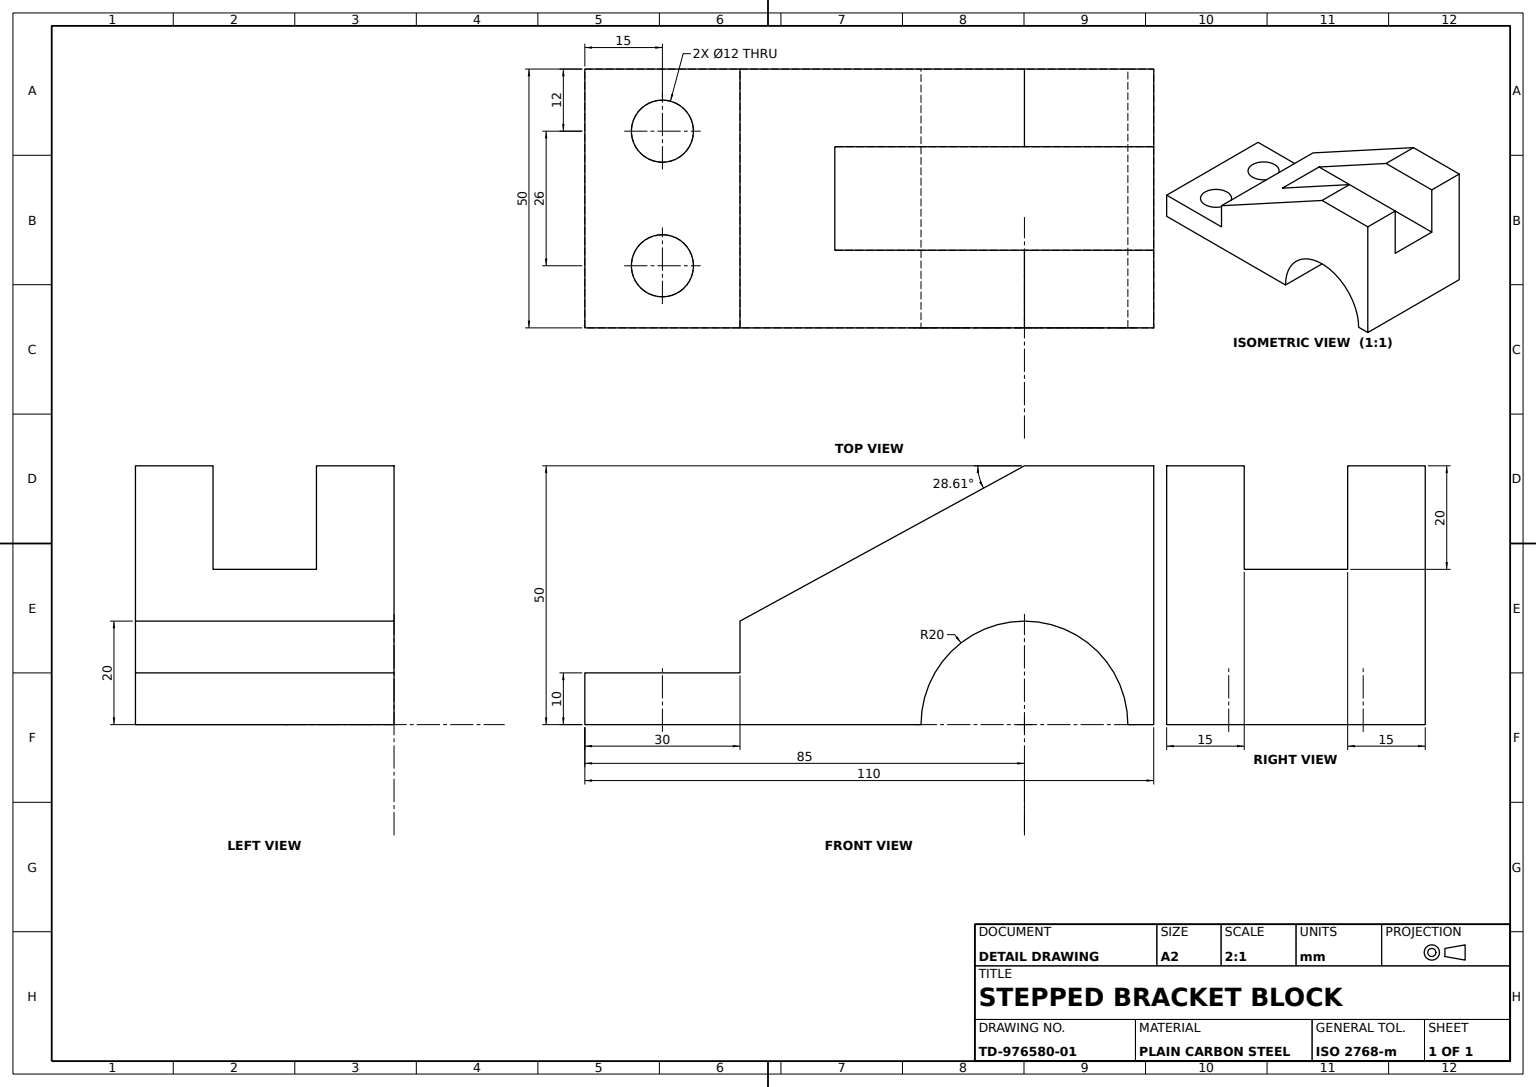
SolidWorks part; units mm, degrees
material "Plain Carbon Steel"
ref_plane "Front Plane" through (0, 0, 0) normal (0, 0, 1) x (1, 0, 0)
ref_plane "Top Plane" through (0, 0, 0) normal (0, 1, 0) x (1, 0, 0)
ref_plane "Right Plane" through (0, 0, 0) normal (1, 0, 0) x (0, 0, -1)
sketch "Bracket Profile Sketch" plane through (0, 0, 0) normal (0, 0, 1) x (1, 0, 0)
  line L0 (0, 0) -> (65, 0)
  line L1 (0, 0) -> (0, 10)
  line L2 (0, 10) -> (30, 10)
  line L3 (105, 0) -> (110, 0)
  line L4 (110, 0) -> (110, 50)
  line L5 (110, 50) -> (85, 50)
  line L6 (30, 10) -> (30, 20)
  line L7 (30, 20) -> (85, 50)
  arc A0 (105, 0) -> (65, 0) centre (85, 0) ccw
  dimension "D1" = 20
  dimension "D2" = 50
  dimension "D3" = 55
  dimension "D4" = 30
  dimension "D5" = 10
  dimension "D6" = 10
  dimension "D7" = 105
  dimension "D8" = 65
  dimension "D9" = 110
extrude "Bracket Body" add sketch "Bracket Profile Sketch" along normal blind 50
sketch "Top Groove Sketch" plane through (0, 50, 0) normal (0, 1, 0) x (1, 0, 0)
  line L0 (110, -50) -> (110, 0) construction
  line L1 (85, -15) -> (110, -15)
  line L2 (85, -15) -> (85, -35)
  line L3 (85, -35) -> (110, -35)
  line L4 (110, -15) -> (110, -35)
  line L5 (85, -15) -> (110, -35) construction
  line L6 (85, -35) -> (110, -15) construction
  line L7 (85, -50) -> (85, 0) construction
  line L8 (110, 0) -> (85, 0) construction
  point P0 (97.5, -25)
  dimension "D1" = 12.5
  dimension "D2" = 15
  dimension "D3" = 25
extrude "Top Groove Cut" cut sketch "Top Groove Sketch" against normal blind 20
sketch "Notch Sketch" plane through (85, 0, 0) normal (1, 0, 0) x (0, 0, -1)
  line L1 (-35, 50) -> (-15, 50)
  line L2 (-35, 50) -> (-35, 30)
  line L3 (-35, 30) -> (-15, 30)
  line L4 (-15, 50) -> (-15, 30)
  line L5 (-35, 50) -> (-15, 30) construction
  line L6 (-35, 30) -> (-15, 50) construction
  point P0 (-25, 40)
extrude "Notch Cut" cut sketch "Notch Sketch" against normal through all
sketch "Mounting Holes Sketch" plane through (0, 10, 0) normal (0, 1, 0) x (1, 0, 0)
  line L0 (0, -50) -> (0, 0) construction
  line L1 (30, 0) -> (0, 0) construction
  circle A0 centre (15, -12) radius 6
  circle A1 centre (15, -38) radius 6
  dimension "D1" = 12
  dimension "D2" = 15
  dimension "D3" = 12
  dimension "D4" = 38
extrude "Mounting Holes 2x" cut sketch "Mounting Holes Sketch" against normal through all
